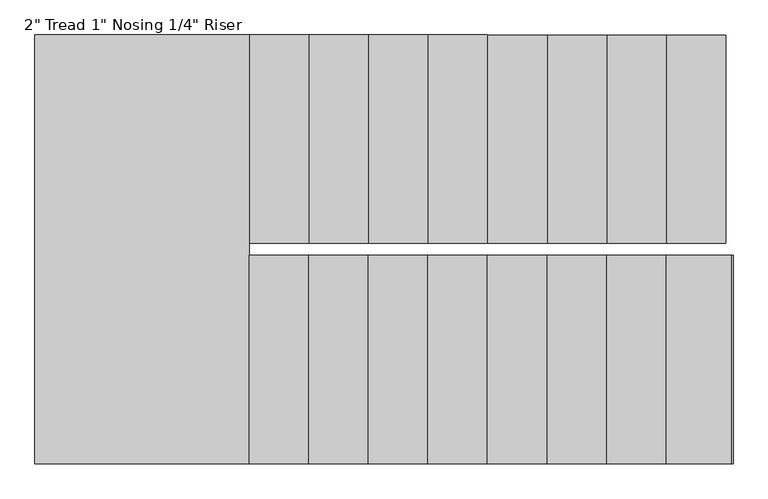
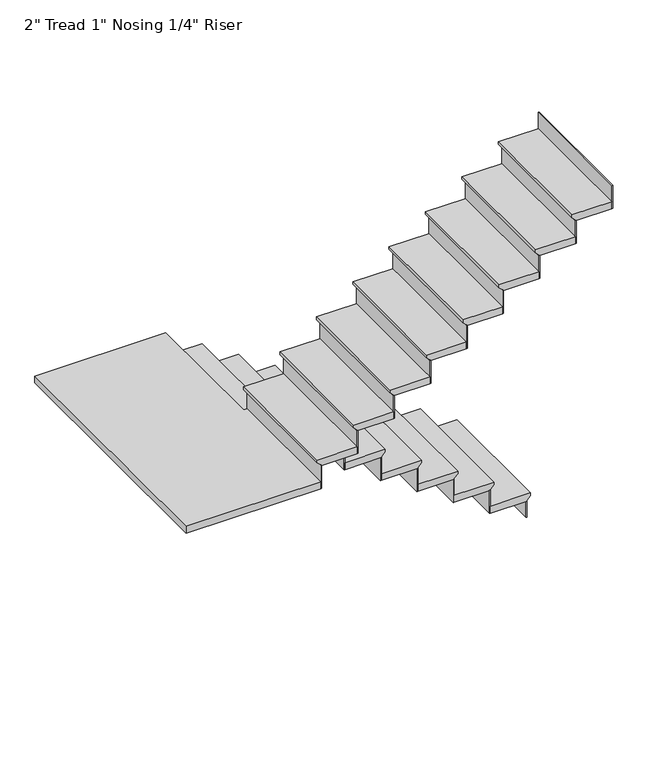
"""IFC4 building model written with IfcOpenShell, lengths in millimetres: stair flight geometry."""

from ifc_helpers import new_model, si_unit, origin, place, context, project, spatial, faceted_brep, source, transform, mapped, element, save


def stair_flight_5a73d723(model_context):
    return source(origin(), model_context, "Body", "Brep", [
        faceted_brep([(-2748.0012202, 5930.6309003, 150.2833333), (-2748.0012202, 5930.6309003, 169.3333333), (-2748.0012202, 5041.6309003, 169.3333333), (-2748.0012202, 5041.6309003, 150.2833333), (-2773.4012202, 5930.6309003, 124.8833333), (-2773.4012202, 5041.6309003, 124.8833333), (-3027.4012202, 5930.6309003, 169.3333333), (-3027.4012202, 5041.6309003, 169.3333333), (-2773.4012202, 5041.6309003, 118.5333333), (-3027.4012202, 5041.6309003, 118.5333333), (-3027.4012202, 5930.6309003, 118.5333333), (-2773.4012202, 5930.6309003, 118.5333333)], [[[0, 1, 2, 3]], [[4, 0, 3, 5]], [[2, 1, 6, 7]], [[8, 9, 10, 11]], [[2, 7, 9, 8, 5, 3]], [[8, 11, 4, 5]], [[6, 1, 0, 4, 11, 10]], [[7, 6, 10, 9]]]),
        faceted_brep([(-2773.4012202, 5930.6309003, 118.5333333), (-2773.4012202, 5930.6309003, 0.0), (-2779.7512202, 5930.6309003, 0.0), (-2779.7512202, 5930.6309003, 118.5333333), (-2773.4012202, 5041.6309003, 118.5333333), (-2779.7512202, 5041.6309003, 118.5333333), (-2779.7512202, 5041.6309003, 0.0), (-2773.4012202, 5041.6309003, 0.0)], [[[0, 1, 2, 3]], [[4, 5, 6, 7]], [[1, 0, 4, 7]], [[2, 1, 7, 6]], [[3, 2, 6, 5]], [[0, 3, 5, 4]]]),
        faceted_brep([(-3027.4012202, 5930.6309003, 287.8666667), (-3027.4012202, 5930.6309003, 118.5333333), (-3033.7512202, 5930.6309003, 118.5333333), (-3033.7512202, 5930.6309003, 287.8666667), (-3027.4012202, 5041.6309003, 287.8666667), (-3033.7512202, 5041.6309003, 287.8666667), (-3033.7512202, 5041.6309003, 118.5333333), (-3027.4012202, 5041.6309003, 118.5333333)], [[[0, 1, 2, 3]], [[4, 5, 6, 7]], [[1, 0, 4, 7]], [[2, 1, 7, 6]], [[3, 2, 6, 5]], [[0, 3, 5, 4]]]),
        faceted_brep([(-3002.0012202, 5041.6309003, 338.6666667), (-3002.0012202, 5930.6309003, 338.6666667), (-3281.4012202, 5930.6309003, 338.6666667), (-3281.4012202, 5041.6309003, 338.6666667), (-3027.4012202, 5041.6309003, 287.8666667), (-3281.4012202, 5041.6309003, 287.8666667), (-3281.4012202, 5930.6309003, 287.8666667), (-3027.4012202, 5930.6309003, 287.8666667), (-3027.4012202, 5041.6309003, 294.2166667), (-3002.0012202, 5041.6309003, 319.6166667), (-3027.4012202, 5930.6309003, 294.2166667), (-3002.0012202, 5930.6309003, 319.6166667)], [[[0, 1, 2, 3]], [[4, 5, 6, 7]], [[0, 3, 5, 4, 8, 9]], [[4, 7, 10, 8]], [[2, 1, 11, 10, 7, 6]], [[3, 2, 6, 5]], [[11, 1, 0, 9]], [[10, 11, 9, 8]]]),
        faceted_brep([(-3281.4012202, 5930.6309003, 457.2), (-3281.4012202, 5930.6309003, 287.8666667), (-3287.7512202, 5930.6309003, 287.8666667), (-3287.7512202, 5930.6309003, 457.2), (-3281.4012202, 5041.6309003, 457.2), (-3287.7512202, 5041.6309003, 457.2), (-3287.7512202, 5041.6309003, 287.8666667), (-3281.4012202, 5041.6309003, 287.8666667)], [[[0, 1, 2, 3]], [[4, 5, 6, 7]], [[1, 0, 4, 7]], [[2, 1, 7, 6]], [[3, 2, 6, 5]], [[0, 3, 5, 4]]]),
        faceted_brep([(-3256.0012202, 5041.6309003, 508.0), (-3256.0012202, 5930.6309003, 508.0), (-3535.4012202, 5930.6309003, 508.0), (-3535.4012202, 5041.6309003, 508.0), (-3281.4012202, 5041.6309003, 457.2), (-3535.4012202, 5041.6309003, 457.2), (-3535.4012202, 5930.6309003, 457.2), (-3281.4012202, 5930.6309003, 457.2), (-3281.4012202, 5041.6309003, 463.55), (-3256.0012202, 5041.6309003, 488.95), (-3281.4012202, 5930.6309003, 463.55), (-3256.0012202, 5930.6309003, 488.95)], [[[0, 1, 2, 3]], [[4, 5, 6, 7]], [[0, 3, 5, 4, 8, 9]], [[4, 7, 10, 8]], [[2, 1, 11, 10, 7, 6]], [[3, 2, 6, 5]], [[11, 1, 0, 9]], [[10, 11, 9, 8]]]),
        faceted_brep([(-3535.4012202, 5930.6309003, 626.5333333), (-3535.4012202, 5930.6309003, 457.2), (-3541.7512202, 5930.6309003, 457.2), (-3541.7512202, 5930.6309003, 626.5333333), (-3535.4012202, 5041.6309003, 626.5333333), (-3541.7512202, 5041.6309003, 626.5333333), (-3541.7512202, 5041.6309003, 457.2), (-3535.4012202, 5041.6309003, 457.2)], [[[0, 1, 2, 3]], [[4, 5, 6, 7]], [[1, 0, 4, 7]], [[2, 1, 7, 6]], [[3, 2, 6, 5]], [[0, 3, 5, 4]]]),
        faceted_brep([(-3510.0012202, 5041.6309003, 677.3333333), (-3510.0012202, 5930.6309003, 677.3333333), (-3789.4012202, 5930.6309003, 677.3333333), (-3789.4012202, 5041.6309003, 677.3333333), (-3535.4012202, 5041.6309003, 626.5333333), (-3789.4012202, 5041.6309003, 626.5333333), (-3789.4012202, 5930.6309003, 626.5333333), (-3535.4012202, 5930.6309003, 626.5333333), (-3535.4012202, 5041.6309003, 632.8833333), (-3510.0012202, 5041.6309003, 658.2833333), (-3535.4012202, 5930.6309003, 632.8833333), (-3510.0012202, 5930.6309003, 658.2833333)], [[[0, 1, 2, 3]], [[4, 5, 6, 7]], [[0, 3, 5, 4, 8, 9]], [[4, 7, 10, 8]], [[2, 1, 11, 10, 7, 6]], [[3, 2, 6, 5]], [[11, 1, 0, 9]], [[10, 11, 9, 8]]]),
        faceted_brep([(-3789.4012202, 5930.6309003, 795.8666667), (-3789.4012202, 5930.6309003, 626.5333333), (-3795.7512202, 5930.6309003, 626.5333333), (-3795.7512202, 5930.6309003, 795.8666667), (-3789.4012202, 5041.6309003, 795.8666667), (-3795.7512202, 5041.6309003, 795.8666667), (-3795.7512202, 5041.6309003, 626.5333333), (-3789.4012202, 5041.6309003, 626.5333333)], [[[0, 1, 2, 3]], [[4, 5, 6, 7]], [[1, 0, 4, 7]], [[2, 1, 7, 6]], [[3, 2, 6, 5]], [[0, 3, 5, 4]]]),
        faceted_brep([(-3764.0012202, 5041.6309003, 846.6666667), (-3764.0012202, 5930.6309003, 846.6666667), (-4043.4012202, 5930.6309003, 846.6666667), (-4043.4012202, 5041.6309003, 846.6666667), (-3789.4012202, 5041.6309003, 795.8666667), (-4043.4012202, 5041.6309003, 795.8666667), (-4043.4012202, 5930.6309003, 795.8666667), (-3789.4012202, 5930.6309003, 795.8666667), (-3789.4012202, 5041.6309003, 802.2166667), (-3764.0012202, 5041.6309003, 827.6166667), (-3789.4012202, 5930.6309003, 802.2166667), (-3764.0012202, 5930.6309003, 827.6166667)], [[[0, 1, 2, 3]], [[4, 5, 6, 7]], [[0, 3, 5, 4, 8, 9]], [[4, 7, 10, 8]], [[2, 1, 11, 10, 7, 6]], [[3, 2, 6, 5]], [[11, 1, 0, 9]], [[10, 11, 9, 8]]]),
        faceted_brep([(-4043.4012202, 5930.6309003, 965.2), (-4043.4012202, 5930.6309003, 795.8666667), (-4049.7512202, 5930.6309003, 795.8666667), (-4049.7512202, 5930.6309003, 965.2), (-4043.4012202, 5041.6309003, 965.2), (-4049.7512202, 5041.6309003, 965.2), (-4049.7512202, 5041.6309003, 795.8666667), (-4043.4012202, 5041.6309003, 795.8666667)], [[[0, 1, 2, 3]], [[4, 5, 6, 7]], [[1, 0, 4, 7]], [[2, 1, 7, 6]], [[3, 2, 6, 5]], [[0, 3, 5, 4]]]),
        faceted_brep([(-4018.0012202, 5041.6309003, 1016.0), (-4018.0012202, 5930.6309003, 1016.0), (-4297.4012202, 5930.6309003, 1016.0), (-4297.4012202, 5041.6309003, 1016.0), (-4043.4012202, 5041.6309003, 965.2), (-4297.4012202, 5041.6309003, 965.2), (-4297.4012202, 5930.6309003, 965.2), (-4043.4012202, 5930.6309003, 965.2), (-4043.4012202, 5041.6309003, 971.55), (-4018.0012202, 5041.6309003, 996.95), (-4043.4012202, 5930.6309003, 971.55), (-4018.0012202, 5930.6309003, 996.95)], [[[0, 1, 2, 3]], [[4, 5, 6, 7]], [[0, 3, 5, 4, 8, 9]], [[4, 7, 10, 8]], [[2, 1, 11, 10, 7, 6]], [[3, 2, 6, 5]], [[11, 1, 0, 9]], [[10, 11, 9, 8]]]),
        faceted_brep([(-4297.4012202, 5930.6309003, 1134.5333333), (-4297.4012202, 5930.6309003, 965.2), (-4303.7512202, 5930.6309003, 965.2), (-4303.7512202, 5930.6309003, 1134.5333333), (-4297.4012202, 5041.6309003, 1134.5333333), (-4303.7512202, 5041.6309003, 1134.5333333), (-4303.7512202, 5041.6309003, 965.2), (-4297.4012202, 5041.6309003, 965.2)], [[[0, 1, 2, 3]], [[4, 5, 6, 7]], [[1, 0, 4, 7]], [[2, 1, 7, 6]], [[3, 2, 6, 5]], [[0, 3, 5, 4]]]),
        faceted_brep([(-4272.0012202, 5041.6309003, 1185.3333333), (-4272.0012202, 5930.6309003, 1185.3333333), (-4551.4012202, 5930.6309003, 1185.3333333), (-4551.4012202, 5041.6309003, 1185.3333333), (-4297.4012202, 5041.6309003, 1134.5333333), (-4551.4012202, 5041.6309003, 1134.5333333), (-4551.4012202, 5930.6309003, 1134.5333333), (-4297.4012202, 5930.6309003, 1134.5333333), (-4297.4012202, 5041.6309003, 1140.8833333), (-4272.0012202, 5041.6309003, 1166.2833333), (-4297.4012202, 5930.6309003, 1140.8833333), (-4272.0012202, 5930.6309003, 1166.2833333)], [[[0, 1, 2, 3]], [[4, 5, 6, 7]], [[0, 3, 5, 4, 8, 9]], [[4, 7, 10, 8]], [[2, 1, 11, 10, 7, 6]], [[3, 2, 6, 5]], [[11, 1, 0, 9]], [[10, 11, 9, 8]]]),
        faceted_brep([(-4551.4012202, 5930.6309003, 1303.8666667), (-4551.4012202, 5930.6309003, 1134.5333333), (-4557.7512202, 5930.6309003, 1134.5333333), (-4557.7512202, 5930.6309003, 1303.8666667), (-4551.4012202, 5041.6309003, 1303.8666667), (-4557.7512202, 5041.6309003, 1303.8666667), (-4557.7512202, 5041.6309003, 1134.5333333), (-4551.4012202, 5041.6309003, 1134.5333333)], [[[0, 1, 2, 3]], [[4, 5, 6, 7]], [[1, 0, 4, 7]], [[2, 1, 7, 6]], [[3, 2, 6, 5]], [[0, 3, 5, 4]]]),
        faceted_brep([(-4526.0012202, 5041.6309003, 1354.6666667), (-4526.0012202, 5930.6309003, 1354.6666667), (-4805.4012202, 5930.6309003, 1354.6666667), (-4805.4012202, 5041.6309003, 1354.6666667), (-4551.4012202, 5041.6309003, 1303.8666667), (-4805.4012202, 5041.6309003, 1303.8666667), (-4805.4012202, 5930.6309003, 1303.8666667), (-4551.4012202, 5930.6309003, 1303.8666667), (-4551.4012202, 5041.6309003, 1310.2166667), (-4526.0012202, 5041.6309003, 1335.6166667), (-4551.4012202, 5930.6309003, 1310.2166667), (-4526.0012202, 5930.6309003, 1335.6166667)], [[[0, 1, 2, 3]], [[4, 5, 6, 7]], [[0, 3, 5, 4, 8, 9]], [[4, 7, 10, 8]], [[2, 1, 11, 10, 7, 6]], [[3, 2, 6, 5]], [[11, 1, 0, 9]], [[10, 11, 9, 8]]]),
        faceted_brep([(-4805.4012202, 5930.6309003, 1473.2), (-4805.4012202, 5930.6309003, 1303.8666667), (-4811.7512202, 5930.6309003, 1303.8666667), (-4811.7512202, 5930.6309003, 1473.2), (-4805.4012202, 5041.6309003, 1473.2), (-4811.7512202, 5041.6309003, 1473.2), (-4811.7512202, 5041.6309003, 1303.8666667), (-4805.4012202, 5041.6309003, 1303.8666667)], [[[0, 1, 2, 3]], [[4, 5, 6, 7]], [[1, 0, 4, 7]], [[2, 1, 7, 6]], [[3, 2, 6, 5]], [[0, 3, 5, 4]]]),
        faceted_brep([(-4754.6012202, 4990.8309003, 1524.0), (-4780.0012202, 4990.8309003, 1524.0), (-4780.0012202, 5930.6309003, 1524.0), (-5694.4012202, 5930.6309003, 1524.0), (-5694.4012202, 4101.8309003, 1524.0), (-4754.6012202, 4101.8309003, 1524.0), (-4780.0012202, 4990.8309003, 1473.2), (-4754.6012202, 4990.8309003, 1473.2), (-4754.6012202, 4101.8309003, 1473.2), (-5694.4012202, 4101.8309003, 1473.2), (-5694.4012202, 5930.6309003, 1473.2), (-4805.4012202, 5930.6309003, 1473.2), (-4805.4012202, 5041.6309003, 1473.2), (-4780.0012202, 5041.6309003, 1473.2), (-4780.0012202, 5041.6309003, 1504.95), (-4780.0012202, 5930.6309003, 1504.95), (-4805.4012202, 5041.6309003, 1479.55), (-4805.4012202, 5930.6309003, 1479.55)], [[[0, 1, 2, 3, 4, 5]], [[6, 7, 8, 9, 10, 11, 12, 13]], [[1, 0, 7, 6]], [[2, 1, 6, 13, 14, 15]], [[13, 12, 16, 14]], [[12, 11, 17, 16]], [[3, 2, 15, 17, 11, 10]], [[4, 3, 10, 9]], [[5, 4, 9, 8]], [[0, 5, 8, 7]], [[17, 15, 14, 16]]]),
        faceted_brep([(-4754.6012202, 4101.8309003, 1642.5333333), (-4754.6012202, 4101.8309003, 1473.2), (-4748.2512202, 4101.8309003, 1473.2), (-4748.2512202, 4101.8309003, 1642.5333333), (-4754.6012202, 4990.8309003, 1642.5333333), (-4748.2512202, 4990.8309003, 1642.5333333), (-4748.2512202, 4990.8309003, 1473.2), (-4754.6012202, 4990.8309003, 1473.2)], [[[0, 1, 2, 3]], [[4, 5, 6, 7]], [[1, 0, 4, 7]], [[2, 1, 7, 6]], [[3, 2, 6, 5]], [[0, 3, 5, 4]]]),
        faceted_brep([(-4780.0012202, 4990.8309003, 1693.3333333), (-4780.0012202, 4101.8309003, 1693.3333333), (-4500.6012202, 4101.8309003, 1693.3333333), (-4500.6012202, 4990.8309003, 1693.3333333), (-4754.6012202, 4990.8309003, 1642.5333333), (-4500.6012202, 4990.8309003, 1642.5333333), (-4500.6012202, 4101.8309003, 1642.5333333), (-4754.6012202, 4101.8309003, 1642.5333333), (-4754.6012202, 4990.8309003, 1648.8833333), (-4780.0012202, 4990.8309003, 1674.2833333), (-4754.6012202, 4101.8309003, 1648.8833333), (-4780.0012202, 4101.8309003, 1674.2833333)], [[[0, 1, 2, 3]], [[4, 5, 6, 7]], [[0, 3, 5, 4, 8, 9]], [[4, 7, 10, 8]], [[2, 1, 11, 10, 7, 6]], [[3, 2, 6, 5]], [[11, 1, 0, 9]], [[10, 11, 9, 8]]]),
        faceted_brep([(-4500.6012202, 4101.8309003, 1811.8666667), (-4500.6012202, 4101.8309003, 1642.5333333), (-4494.2512202, 4101.8309003, 1642.5333333), (-4494.2512202, 4101.8309003, 1811.8666667), (-4500.6012202, 4990.8309003, 1811.8666667), (-4494.2512202, 4990.8309003, 1811.8666667), (-4494.2512202, 4990.8309003, 1642.5333333), (-4500.6012202, 4990.8309003, 1642.5333333)], [[[0, 1, 2, 3]], [[4, 5, 6, 7]], [[1, 0, 4, 7]], [[2, 1, 7, 6]], [[3, 2, 6, 5]], [[0, 3, 5, 4]]]),
        faceted_brep([(-4526.0012202, 4990.8309003, 1862.6666667), (-4526.0012202, 4101.8309003, 1862.6666667), (-4246.6012202, 4101.8309003, 1862.6666667), (-4246.6012202, 4990.8309003, 1862.6666667), (-4500.6012202, 4990.8309003, 1811.8666667), (-4246.6012202, 4990.8309003, 1811.8666667), (-4246.6012202, 4101.8309003, 1811.8666667), (-4500.6012202, 4101.8309003, 1811.8666667), (-4500.6012202, 4990.8309003, 1818.2166667), (-4526.0012202, 4990.8309003, 1843.6166667), (-4500.6012202, 4101.8309003, 1818.2166667), (-4526.0012202, 4101.8309003, 1843.6166667)], [[[0, 1, 2, 3]], [[4, 5, 6, 7]], [[0, 3, 5, 4, 8, 9]], [[4, 7, 10, 8]], [[2, 1, 11, 10, 7, 6]], [[3, 2, 6, 5]], [[11, 1, 0, 9]], [[10, 11, 9, 8]]]),
        faceted_brep([(-4246.6012202, 4101.8309003, 1981.2), (-4246.6012202, 4101.8309003, 1811.8666667), (-4240.2512202, 4101.8309003, 1811.8666667), (-4240.2512202, 4101.8309003, 1981.2), (-4246.6012202, 4990.8309003, 1981.2), (-4240.2512202, 4990.8309003, 1981.2), (-4240.2512202, 4990.8309003, 1811.8666667), (-4246.6012202, 4990.8309003, 1811.8666667)], [[[0, 1, 2, 3]], [[4, 5, 6, 7]], [[1, 0, 4, 7]], [[2, 1, 7, 6]], [[3, 2, 6, 5]], [[0, 3, 5, 4]]]),
        faceted_brep([(-4272.0012202, 4990.8309003, 2032.0), (-4272.0012202, 4101.8309003, 2032.0), (-3992.6012202, 4101.8309003, 2032.0), (-3992.6012202, 4990.8309003, 2032.0), (-4246.6012202, 4990.8309003, 1981.2), (-3992.6012202, 4990.8309003, 1981.2), (-3992.6012202, 4101.8309003, 1981.2), (-4246.6012202, 4101.8309003, 1981.2), (-4246.6012202, 4990.8309003, 1987.55), (-4272.0012202, 4990.8309003, 2012.95), (-4246.6012202, 4101.8309003, 1987.55), (-4272.0012202, 4101.8309003, 2012.95)], [[[0, 1, 2, 3]], [[4, 5, 6, 7]], [[0, 3, 5, 4, 8, 9]], [[4, 7, 10, 8]], [[2, 1, 11, 10, 7, 6]], [[3, 2, 6, 5]], [[11, 1, 0, 9]], [[10, 11, 9, 8]]]),
        faceted_brep([(-3992.6012202, 4101.8309003, 2150.5333333), (-3992.6012202, 4101.8309003, 1981.2), (-3986.2512202, 4101.8309003, 1981.2), (-3986.2512202, 4101.8309003, 2150.5333333), (-3992.6012202, 4990.8309003, 2150.5333333), (-3986.2512202, 4990.8309003, 2150.5333333), (-3986.2512202, 4990.8309003, 1981.2), (-3992.6012202, 4990.8309003, 1981.2)], [[[0, 1, 2, 3]], [[4, 5, 6, 7]], [[1, 0, 4, 7]], [[2, 1, 7, 6]], [[3, 2, 6, 5]], [[0, 3, 5, 4]]]),
        faceted_brep([(-4018.0012202, 4990.8309003, 2201.3333333), (-4018.0012202, 4101.8309003, 2201.3333333), (-3738.6012202, 4101.8309003, 2201.3333333), (-3738.6012202, 4990.8309003, 2201.3333333), (-3992.6012202, 4990.8309003, 2150.5333333), (-3738.6012202, 4990.8309003, 2150.5333333), (-3738.6012202, 4101.8309003, 2150.5333333), (-3992.6012202, 4101.8309003, 2150.5333333), (-3992.6012202, 4990.8309003, 2156.8833333), (-4018.0012202, 4990.8309003, 2182.2833333), (-3992.6012202, 4101.8309003, 2156.8833333), (-4018.0012202, 4101.8309003, 2182.2833333)], [[[0, 1, 2, 3]], [[4, 5, 6, 7]], [[0, 3, 5, 4, 8, 9]], [[4, 7, 10, 8]], [[2, 1, 11, 10, 7, 6]], [[3, 2, 6, 5]], [[11, 1, 0, 9]], [[10, 11, 9, 8]]]),
        faceted_brep([(-3738.6012202, 4101.8309003, 2319.8666667), (-3738.6012202, 4101.8309003, 2150.5333333), (-3732.2512202, 4101.8309003, 2150.5333333), (-3732.2512202, 4101.8309003, 2319.8666667), (-3738.6012202, 4990.8309003, 2319.8666667), (-3732.2512202, 4990.8309003, 2319.8666667), (-3732.2512202, 4990.8309003, 2150.5333333), (-3738.6012202, 4990.8309003, 2150.5333333)], [[[0, 1, 2, 3]], [[4, 5, 6, 7]], [[1, 0, 4, 7]], [[2, 1, 7, 6]], [[3, 2, 6, 5]], [[0, 3, 5, 4]]]),
        faceted_brep([(-3764.0012202, 4990.8309003, 2370.6666667), (-3764.0012202, 4101.8309003, 2370.6666667), (-3484.6012202, 4101.8309003, 2370.6666667), (-3484.6012202, 4990.8309003, 2370.6666667), (-3738.6012202, 4990.8309003, 2319.8666667), (-3484.6012202, 4990.8309003, 2319.8666667), (-3484.6012202, 4101.8309003, 2319.8666667), (-3738.6012202, 4101.8309003, 2319.8666667), (-3738.6012202, 4990.8309003, 2326.2166667), (-3764.0012202, 4990.8309003, 2351.6166667), (-3738.6012202, 4101.8309003, 2326.2166667), (-3764.0012202, 4101.8309003, 2351.6166667)], [[[0, 1, 2, 3]], [[4, 5, 6, 7]], [[0, 3, 5, 4, 8, 9]], [[4, 7, 10, 8]], [[2, 1, 11, 10, 7, 6]], [[3, 2, 6, 5]], [[11, 1, 0, 9]], [[10, 11, 9, 8]]]),
        faceted_brep([(-3484.6012202, 4101.8309003, 2489.2), (-3484.6012202, 4101.8309003, 2319.8666667), (-3478.2512202, 4101.8309003, 2319.8666667), (-3478.2512202, 4101.8309003, 2489.2), (-3484.6012202, 4990.8309003, 2489.2), (-3478.2512202, 4990.8309003, 2489.2), (-3478.2512202, 4990.8309003, 2319.8666667), (-3484.6012202, 4990.8309003, 2319.8666667)], [[[0, 1, 2, 3]], [[4, 5, 6, 7]], [[1, 0, 4, 7]], [[2, 1, 7, 6]], [[3, 2, 6, 5]], [[0, 3, 5, 4]]]),
        faceted_brep([(-3510.0012202, 4990.8309003, 2540.0), (-3510.0012202, 4101.8309003, 2540.0), (-3230.6012202, 4101.8309003, 2540.0), (-3230.6012202, 4990.8309003, 2540.0), (-3484.6012202, 4990.8309003, 2489.2), (-3230.6012202, 4990.8309003, 2489.2), (-3230.6012202, 4101.8309003, 2489.2), (-3484.6012202, 4101.8309003, 2489.2), (-3484.6012202, 4990.8309003, 2495.55), (-3510.0012202, 4990.8309003, 2520.95), (-3484.6012202, 4101.8309003, 2495.55), (-3510.0012202, 4101.8309003, 2520.95)], [[[0, 1, 2, 3]], [[4, 5, 6, 7]], [[0, 3, 5, 4, 8, 9]], [[4, 7, 10, 8]], [[2, 1, 11, 10, 7, 6]], [[3, 2, 6, 5]], [[11, 1, 0, 9]], [[10, 11, 9, 8]]]),
        faceted_brep([(-3230.6012202, 4101.8309003, 2658.5333333), (-3230.6012202, 4101.8309003, 2489.2), (-3224.2512202, 4101.8309003, 2489.2), (-3224.2512202, 4101.8309003, 2658.5333333), (-3230.6012202, 4990.8309003, 2658.5333333), (-3224.2512202, 4990.8309003, 2658.5333333), (-3224.2512202, 4990.8309003, 2489.2), (-3230.6012202, 4990.8309003, 2489.2)], [[[0, 1, 2, 3]], [[4, 5, 6, 7]], [[1, 0, 4, 7]], [[2, 1, 7, 6]], [[3, 2, 6, 5]], [[0, 3, 5, 4]]]),
        faceted_brep([(-3256.0012202, 4990.8309003, 2709.3333333), (-3256.0012202, 4101.8309003, 2709.3333333), (-2976.6012202, 4101.8309003, 2709.3333333), (-2976.6012202, 4990.8309003, 2709.3333333), (-3230.6012202, 4990.8309003, 2658.5333333), (-2976.6012202, 4990.8309003, 2658.5333333), (-2976.6012202, 4101.8309003, 2658.5333333), (-3230.6012202, 4101.8309003, 2658.5333333), (-3230.6012202, 4990.8309003, 2664.8833333), (-3256.0012202, 4990.8309003, 2690.2833333), (-3230.6012202, 4101.8309003, 2664.8833333), (-3256.0012202, 4101.8309003, 2690.2833333)], [[[0, 1, 2, 3]], [[4, 5, 6, 7]], [[0, 3, 5, 4, 8, 9]], [[4, 7, 10, 8]], [[2, 1, 11, 10, 7, 6]], [[3, 2, 6, 5]], [[11, 1, 0, 9]], [[10, 11, 9, 8]]]),
        faceted_brep([(-2976.6012202, 4101.8309003, 2827.8666667), (-2976.6012202, 4101.8309003, 2658.5333333), (-2970.2512202, 4101.8309003, 2658.5333333), (-2970.2512202, 4101.8309003, 2827.8666667), (-2976.6012202, 4990.8309003, 2827.8666667), (-2970.2512202, 4990.8309003, 2827.8666667), (-2970.2512202, 4990.8309003, 2658.5333333), (-2976.6012202, 4990.8309003, 2658.5333333)], [[[0, 1, 2, 3]], [[4, 5, 6, 7]], [[1, 0, 4, 7]], [[2, 1, 7, 6]], [[3, 2, 6, 5]], [[0, 3, 5, 4]]]),
        faceted_brep([(-2722.6012202, 4101.8309003, 2997.2), (-2722.6012202, 4101.8309003, 2827.8666667), (-2716.2512202, 4101.8309003, 2827.8666667), (-2716.2512202, 4101.8309003, 2997.2), (-2722.6012202, 4990.8309003, 2997.2), (-2716.2512202, 4990.8309003, 2997.2), (-2716.2512202, 4990.8309003, 2827.8666667), (-2722.6012202, 4990.8309003, 2827.8666667)], [[[0, 1, 2, 3]], [[4, 5, 6, 7]], [[1, 0, 4, 7]], [[2, 1, 7, 6]], [[3, 2, 6, 5]], [[0, 3, 5, 4]]]),
        faceted_brep([(-3002.0012202, 4990.8309003, 2878.6666667), (-3002.0012202, 4101.8309003, 2878.6666667), (-2722.6012202, 4101.8309003, 2878.6666667), (-2722.6012202, 4990.8309003, 2878.6666667), (-2976.6012202, 4990.8309003, 2827.8666667), (-2722.6012202, 4990.8309003, 2827.8666667), (-2722.6012202, 4101.8309003, 2827.8666667), (-2976.6012202, 4101.8309003, 2827.8666667), (-2976.6012202, 4990.8309003, 2834.2166667), (-3002.0012202, 4990.8309003, 2859.6166667), (-2976.6012202, 4101.8309003, 2834.2166667), (-3002.0012202, 4101.8309003, 2859.6166667)], [[[0, 1, 2, 3]], [[4, 5, 6, 7]], [[0, 3, 5, 4, 8, 9]], [[4, 7, 10, 8]], [[2, 1, 11, 10, 7, 6]], [[3, 2, 6, 5]], [[11, 1, 0, 9]], [[10, 11, 9, 8]]]),
    ])


if __name__ == "__main__":
    model = new_model("IFC4")
    model_context = context("Model", 3, world=origin())
    ifc_project = project(units=[si_unit("LENGTHUNIT", "METRE", prefix="MILLI")], contexts=[model_context])
    site = spatial("IfcSite", under=ifc_project)
    building = spatial("IfcBuilding", under=site)
    placement = place(None, origin())
    stair_flight_shape = stair_flight_5a73d723(model_context)
    element("IfcStairFlight", 1, ObjectType="2\" Tread 1\" Nosing 1/4\" Riser", at=placement, inside=building, context=model_context, shape_type="MappedRepresentation", body=[
        mapped(stair_flight_shape, transform((0.0, 0.0, 0.0), x_axis=(1.0, 0.0, 0.0), y_axis=(0.0, 1.0, 0.0), z_axis=(0.0, 0.0, 1.0))),
    ])
    save(model, "model.ifc")
